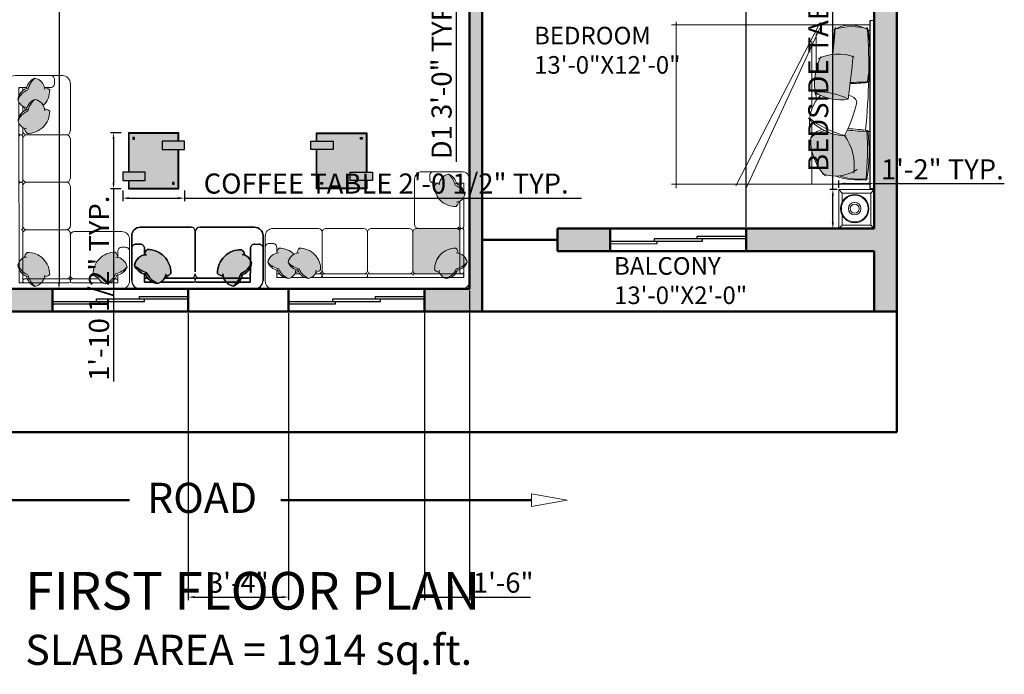
# Model space of a CAD drawing. Units: inches. Extents: x 1913 to 5309, y 1003 to 1733.
# Tile 10 of 23: x 2850 to 3242, y 1003 to 1263. Entities that reach past the tile are written whole.
import ezdxf

# ---------------------------------------------------------------- set-up
doc = ezdxf.new("R2010")
doc.units = ezdxf.units.IN
for name, color, linetype, lineweight in [('0.10', 252, 'Continuous', 9), ('0.15', 34, 'Continuous', 15), ('A-ANNO-DIMS', 2, 'Continuous', 18), ('A-ANNO-SYMB', 1, 'Continuous', 18), ('A-ANNO-TEXT', 7, 'Continuous', 18), ('A-AREA-IDEN', 3, 'Continuous', 18), ('A-DOOR', 4, 'Continuous', 25), ('A-FLOR-PATT', 252, 'Continuous', 13), ('A-FURN', 8, 'Continuous', 18), ('A-FURN-PATT', 8, 'Continuous', 13), ('A-GLAZ', 5, 'Continuous', 25), ('A-WALL', 7, 'Continuous', 50)]:
    doc.layers.add(name, color=color, linetype=linetype, lineweight=lineweight)
doc.layers.add('MOBIL', color=7, linetype='Continuous')
doc.styles.get("Standard").update_dxf_attribs({"font": 'arial.ttf'})
doc.dimstyles.new('ISO-25', dxfattribs={"dimtxt": 8, "dimasz": 2.5, "dimexe": 1.25, "dimexo": 0.625, "dimtad": 1, "dimdec": 1, "dimlunit": 3, "dimtxsty": 'Standard', "dimcen": 2.5, "dimclrd": 256, "dimclrt": 1, "dimadec": 0, "dimazin": 0, "dimtfac": 1, "dimtdec": 1, "dimtmove": 0, "dimatfit": 3, "dimfxl": 1, "dimarcsym": 0})

# ---------------------------------------------------------------- blocks, each defined once
blk = doc.blocks.new('Mesa de centro Cantria feeling')
at = {"layer": 'MOBIL', "ltscale": 0.2}
h = blk.add_hatch(color=256, dxfattribs=at)
h.set_gradient(color1=(74, 55, 38), color2=(104, 77, 54), one_color=1, tint=0.31, name='CYLINDER')
h.paths.add_polyline_path([(-0.85, -0.3), (-0.7, -0.3), (-0.7, 0.1), (-0.85, 0.1)])
h = blk.add_hatch(color=256, dxfattribs=at)
h.set_gradient(color1=(221, 221, 223), one_color=1, tint=1)
h.paths.add_polyline_path([(-0.15, -0.6), (-0.15, -0.89), (-0.01, -0.89), (-0.01, -0.01), (-0.7, -0.01), (-0.7, -0.3), (-0.85, -0.3), (-0.85, -0.01), (-0.99, -0.01), (-0.99, -0.89), (-0.3, -0.89), (-0.3, -0.6)])
h.paths.add_polyline_path([(-0.112, -0.112), (-0.112, -0.082), (-0.082, -0.082), (-0.082, -0.112)], flags=16)
h.paths.add_polyline_path([(-0.888, -0.788), (-0.888, -0.818), (-0.918, -0.818), (-0.918, -0.788)], flags=16)
h = blk.add_hatch(color=256, dxfattribs=at)
h.set_gradient(color1=(74, 55, 38), color2=(104, 77, 54), one_color=1, tint=0.31, name='CYLINDER')
h.paths.add_polyline_path([(-0.15, -0.6), (-0.3, -0.6), (-0.3, -1), (-0.15, -1)])
for points in [[(-0.85, 0), (-1, 0), (-1, -0.9), (-0.3, -0.9)], [(-0.15, -0.9), (0, -0.9), (0, 0), (-0.7, 0)], [(-0.85, -0.01), (-0.99, -0.01), (-0.99, -0.89), (-0.3, -0.89)], [(-0.15, -0.89), (-0.01, -0.89), (-0.01, -0.01), (-0.7, -0.01)]]:
    blk.add_lwpolyline(points, dxfattribs=at)
for points in [[(-0.85, -0.3), (-0.7, -0.3), (-0.7, 0.1), (-0.85, 0.1)], [(-0.082, -0.082), (-0.112, -0.082), (-0.112, -0.112), (-0.082, -0.112)], [(-0.15, -0.6), (-0.3, -0.6), (-0.3, -1), (-0.15, -1)], [(-0.918, -0.818), (-0.888, -0.818), (-0.888, -0.788), (-0.918, -0.788)]]:
    blk.add_lwpolyline(points, close=True, dxfattribs=at)
blk = doc.blocks.new('camita')
at = {"layer": '0.10'}
for p, q in [((-0.85, -0.045), (0.85, -0.045)), ((-0.805, -0.045), (-0.805, -2.0485)), ((0.805, -0.045), (0.805, -2.0485)), ((-0.8271, -0.521), (0.8464, -1.2932)), ((-0.8271, -0.5476), (0.8236, -1.3992)), ((-0.7161, -0.585), (-0.3554, -0.585)), ((-0.1136, -0.585), (-0.0485, -0.585)), ((-0.638, -0.63), (0.0434, -0.63)), ((0.1749, -0.63), (0.3179, -0.63)), ((0.4739, -0.63), (0.805, -0.63)), ((-0.8354, -2), (0.8464, -2))]:
    blk.add_line(p, q, dxfattribs=at)
blk.add_lwpolyline([(-0.85, -0.0405), (0.85, -0.0405), (0.85, 0), (-0.85, 0)], close=True, dxfattribs=at)
for centre, radius, start, end in [((-0.4574, -0.2364), 0.3443, 147.50996, 213.83359), ((-0.1997, -0.2266), 0.5864, 163.92635, 197.14087), ((-0.3639, -5.8457), 5.7909, 83.80731, 94.12107), ((-0.5104, -1.7232), 1.6781, 80.12554, 98.66187), ((2.3534, -0.0532), 2.5803, 180.10628, 184.38541), ((-1.5443, -0.2452), 1.3333, 359.93941, 7.55329), ((1.5815, -0.2893), 1.3353, 170.38021, 178.99138), ((-1.4396, -0.0609), 1.7117, 352.92911, 0.39592), ((0.4524, -3.0675), 2.9996, 83.90257, 93.67595), ((0.4863, -1.6286), 1.5781, 80.16015, 98.05996), ((0.0294, -0.1377), 0.7262, 342.58415, 6.00484), ((0.1326, -0.1696), 0.6307, 339.92303, 8.74334), ((-0.007, -0.258), 0.0828, 100.01798, 179.73597), ((-0.2931, -1.4378), 1.2903, 61.97485, 77.84351), ((0.3203, -0.3944), 0.4043, 341.45245, 33.45121), ((-0.0543, -0.3633), 0.4542, 159.30257, 206.50263), ((-1.3301, -9.6748), 9.4985, 82.27078, 84.93989), ((0.4585, -0.5454), 0.5842, 151.04555, 184.14969), ((-0.5341, -0.3393), 0.4875, 327.26442, 9.0473), ((-0.1986, -0.2742), 0.5159, 310.73945, 359.05759), ((0.6265, -0.7518), 0.5508, 82.96906, 124.67388), ((-1.8672, -14.986), 14.6323, 84.65974, 85.75157), ((-0.5673, -0.0868), 0.9057, 321.69527, 346.46261), ((-0.4598, 1.4861), 1.9092, 260.95299, 268.65169), ((0.3612, -0.133), 0.5096, 267.25889, 315.29965), ((-0.2002, 0.064), 0.6673, 244.78094, 279.06058), ((0.179, -0.272), 0.3828, 224.52836, 275.22287), ((0.4384, -0.4834), 0.1898, 193.68485, 236.70352), ((0.5707, -0.4317), 0.3145, 192.93877, 221.96363)]:
    blk.add_arc(centre, radius, start, end, dxfattribs=at)
blk = doc.blocks.new('VELADOR')
at = {"layer": '0.15'}
for p, q in [((-0.248, 0), (-0.203, -0.045)), ((0.248, 0), (0.202, -0.045)), ((-0.203, -0.405), (-0.248, -0.45)), ((0.248, -0.45), (0.202, -0.405))]:
    blk.add_line(p, q, dxfattribs=at)
blk.add_lwpolyline([(-0.248, 0), (-0.248, -0.45), (0.248, -0.45), (0.248, 0)], close=True, dxfattribs=at)
blk.add_lwpolyline([(0.092, -0.405), (0.202, -0.405), (0.202, -0.045), (-0.203, -0.045), (-0.203, -0.405), (-0.082, -0.405)], dxfattribs=at)
for radius in [0.18, 0.169, 0.0788, 0.0563]:
    blk.add_circle((0.005, -0.247), radius, dxfattribs=at)
blk = doc.blocks.new('d2 s')
at = {"transparency": 33554687}
h = blk.add_hatch(color=256, dxfattribs=at)
h.dxf.hatch_style = 1
h.paths.add_polyline_path([(3953.01, 1202.6, 0.213835), (3948.73, 1198.21, 0.233217), (3951.28, 1195.23, 0.122039), (3952.62, 1192.95, 0.425972), (3962.37, 1202.51, 0.156703), (3960.25, 1203.55), (3960.12, 1203.55, 0.310469), (3955.94, 1207.57, 0.147724)])
h = blk.add_hatch(color=256, dxfattribs=at)
h.dxf.hatch_style = 1
h.paths.add_polyline_path([(3953.9, 1162.75, -0.084911), (3952.59, 1164.92, -0.046133), (3950.85, 1165.51), (3950.85, 1171.8, -0.039409), (3951.63, 1172.02, -0.165523), (3952.68, 1174.28, -0.42585), (3962.24, 1164.53, -0.121928), (3959.96, 1163.19, -0.027403), (3959.75, 1162.75)])
h.paths.add_polyline_path([(3949.17, 1166.48), (3949.17, 1170.75, -0.097704), (3950.85, 1171.8), (3950.85, 1165.51, -0.04873)])
h.paths.add_polyline_path([(3947.62, 1167.84, -0.16488), (3949.17, 1170.75), (3949.17, 1166.48, -0.051917)])
h.paths.add_polyline_path([(3956, 1161.07, -0.090388), (3953.9, 1162.75), (3959.75, 1162.75, -0.136035), (3958.07, 1161.07)])
blk.add_line((3946.53, 1205.25), (3946.53, 1159.36), dxfattribs=at)
for p, q in [((3949.84, 1161.07), (3950.18, 1161.07)), ((3964.47, 1159.37), (3964.46, 1157.65))]:
    blk.add_line(p, q)
for points in [[(3955.94, 1207.57, 0.147724), (3953.01, 1202.6, 0.213355), (3948.73, 1198.22, -0.213355), (3953.01, 1202.6, -0.147724), (3955.94, 1207.57, 0.249545), (3952.4, 1203.17, -0.249545), (3955.93, 1207.59, -0.356779), (3960.22, 1202.7, 0.356779), (3955.94, 1207.57)], [(3948.72, 1198.23, 0.306333), (3952.42, 1194.91, -0.306333), (3948.72, 1198.23, -0.306674), (3952.79, 1203.29, 0.306674), (3948.72, 1198.23)], [(3952.62, 1192.95, 0.425972), (3962.37, 1202.51, 0.165552), (3960.12, 1203.57, -0.165552), (3962.37, 1202.51, -0.425972), (3952.63, 1192.95, -0.121514), (3951.29, 1195.22, 0.121514), (3952.62, 1192.95)], [(3962.24, 1164.53, 0.425972), (3952.68, 1174.28, 0.165552), (3951.63, 1172.02, -0.165552), (3952.68, 1174.28, -0.425972), (3962.24, 1164.53, -0.121514), (3959.97, 1163.19, 0.121514), (3962.24, 1164.53)], [(3947.62, 1167.84, 0.147724), (3952.59, 1164.92, 0.213355), (3956.97, 1160.64, -0.213355), (3952.59, 1164.92, -0.147724), (3947.62, 1167.84, 0.249545), (3952.02, 1164.3, -0.249545), (3947.61, 1167.84, -0.356779), (3952.49, 1172.13, 0.356779), (3947.62, 1167.84)], [(3956.96, 1160.63, 0.306333), (3960.28, 1164.33, -0.306333), (3956.96, 1160.63, -0.306674), (3951.9, 1164.7, 0.306674), (3956.96, 1160.63)]]:
    blk.add_lwpolyline(points, format="xyb", dxfattribs=at)
for points in [[(3949.93, 1208.66), (3967.86, 1208.66)], [(3964.46, 1205.25), (3964.46, 1206.96)], [(3971.27, 1205.25), (3971.27, 1184.84)], [(3949.17, 1203.55), (3952.49, 1203.55), (3949.17, 1203.55), (3949.17, 1199.96)], [(3950.85, 1202.87), (3950.85, 1202.25)], [(3960.13, 1203.55), (3962.77, 1203.55)], [(3949.17, 1197.14), (3949.17, 1183.83)], [(3950.85, 1195.43), (3950.85, 1183.83)], [(3949.17, 1164.09), (3949.17, 1182.51)], [(3950.99, 1183.17), (3950.65, 1183.17)], [(3950.85, 1161.74), (3950.85, 1182.51)], [(3969.63, 1183.17), (3953.36, 1183.17)], [(3971.25, 1181.39), (3971.25, 1159.35)], [(3949.17, 1161.07), (3949.17, 1164.4), (3949.17, 1161.07), (3952.75, 1161.07)], [(3952.75, 1161.06), (3962.77, 1161.06)], [(3949.93, 1155.95), (3967.86, 1155.95)]]:
    blk.add_lwpolyline(points, close=True, dxfattribs=at)
for points in [[(3962.76, 1208.66, -0.414214), (3964.46, 1206.97, 0.414214)], [(3964.46, 1205.26, -0.414214), (3962.76, 1203.57, 0.414214)], [(3967.85, 1208.66, -0.414212), (3971.25, 1205.26, 0.414212)], [(3950.18, 1203.55, -0.414214), (3950.85, 1202.88, 0.414214)], [(3964.47, 1159.37, 0.414214), (3962.77, 1161.06, -0.414214)], [(3967.85, 1155.95, 0.414212), (3971.25, 1159.35, -0.414212)], [(3962.76, 1155.95, 0.414214), (3964.46, 1157.65, -0.414214)]]:
    blk.add_lwpolyline(points, format="xyb", close=True, dxfattribs=at)
for centre, radius, start, end in [((3949.93, 1205.26), 3.4, 90.0002, 179.9998), ((3949.93, 1205.26), 3.4, 90.0846, 180.0842), ((3949.85, 1183.85), 0.681, 179.1575, 269.1575), ((3949.85, 1182.49), 0.681, 90.8425, 180.8425), ((3950.18, 1183.84), 0.671, 270, 0), ((3950.18, 1183.84), 0.671, 270, 0), ((3950.18, 1182.5), 0.671, 360, 90), ((3950.18, 1182.5), 0.671, 360, 90), ((3952.51, 1184.83), 1.66, 179.4889, 271.234), ((3952.51, 1181.52), 1.66, 88.766, 180.5111), ((3969.59, 1184.83), 1.66, 268.766, 0.5111), ((3969.39, 1181.32), 1.86, 2.0577, 84.9818), ((3969.39, 1181.32), 1.86, 2.0577, 84.9818), ((3969.59, 1184.83), 1.66, 268.7816, 0.5111), ((3949.84, 1161.74), 0.671, 180, 270), ((3950.18, 1161.74), 0.671, 270, 0), ((3949.93, 1159.36), 3.4, 180.0002, 269.9998), ((3949.93, 1159.37), 3.4, 180.0846, 270.0842)]:
    blk.add_arc(centre, radius, start, end, dxfattribs=at)
blk = doc.blocks.new('SOFA 1')
at = {"transparency": 33554687}
h = blk.add_hatch(color=256, dxfattribs=at)
h.dxf.hatch_style = 1
h.paths.add_polyline_path([(3769.65, 1307.6, 0.084911), (3767.15, 1309.12, 0.046133), (3766.46, 1311.13), (3759.18, 1311.13, 0.039409), (3758.92, 1310.24, 0.165523), (3756.31, 1309.02, 0.42585), (3767.59, 1297.95, 0.121928), (3769.15, 1300.58, 0.027403), (3769.65, 1300.83)])
h.paths.add_polyline_path([(3765.34, 1313.08), (3760.4, 1313.08, 0.097704), (3759.18, 1311.13), (3766.46, 1311.13, 0.04873)])
h.paths.add_polyline_path([(3763.76, 1314.88, 0.16488), (3760.4, 1313.08), (3765.34, 1313.08, 0.051917)])
h.paths.add_polyline_path([(3771.6, 1305.17, 0.090388), (3769.65, 1307.6), (3769.65, 1300.83, 0.136035), (3771.6, 1302.77)])
h = blk.add_hatch(color=256, dxfattribs=at)
h.dxf.hatch_style = 1
h.paths.add_polyline_path([(3723.52, 1308.63, 0.147724), (3717.76, 1305.24, 0.310469), (3722.42, 1300.4), (3722.42, 1300.25, 0.156703), (3723.62, 1297.8, 0.425821), (3734.69, 1309.08, 0.121928), (3732.05, 1310.63, 0.233216), (3728.6, 1313.59, 0.213835)])
h = blk.add_hatch(color=256, dxfattribs=at)
h.dxf.hatch_style = 1
h.paths.add_polyline_path([(3769.16, 1235.96, 0.122267), (3767.6, 1238.61, 0.425972), (3756.32, 1227.54, 0.165563), (3758.93, 1226.32, 0.309481), (3763.76, 1221.69, 0.002677), (3763.83, 1221.72, 0.146094), (3767.16, 1227.43, 0.212433), (3772.1, 1232.48, 0.235342)])
h = blk.add_hatch(color=256, dxfattribs=at)
h.dxf.hatch_style = 1
h.paths.add_polyline_path([(3769.16, 1225.36, 0.122267), (3767.6, 1228.01, 0.425972), (3756.32, 1216.94, 0.165563), (3758.93, 1215.72, 0.309481), (3763.76, 1211.09, 0.002677), (3763.83, 1211.12, 0.146094), (3767.16, 1216.83, 0.212433), (3772.1, 1221.88, 0.235342)])
for p, q in [((3720.45, 1316.13), (3773.58, 1316.13)), ((3777.51, 1312.19), (3777.51, 1213.72))]:
    blk.add_line(p, q, dxfattribs=at)
for points in [[(3763.76, 1314.88, -0.147724), (3767.15, 1309.12, -0.213355), (3772.1, 1304.05, 0.213355), (3767.15, 1309.12, 0.147724), (3763.76, 1314.88, -0.249545), (3767.86, 1309.77, 0.249545), (3763.77, 1314.89, 0.356779), (3758.8, 1309.23, -0.356779), (3763.76, 1314.88)], [(3717.76, 1305.24, -0.147724), (3723.52, 1308.63, -0.213355), (3728.59, 1313.59, 0.213355), (3723.52, 1308.63, 0.147724), (3717.76, 1305.24, -0.249545), (3722.86, 1309.34, 0.249545), (3717.75, 1305.25, 0.356779), (3723.4, 1300.28, -0.356779), (3717.76, 1305.24)], [(3734.69, 1309.08, -0.425972), (3723.62, 1297.8, -0.165552), (3722.4, 1300.4, 0.165552), (3723.62, 1297.79, 0.425972), (3734.69, 1309.07, 0.121514), (3732.07, 1310.63, -0.121514), (3734.69, 1309.08)], [(3728.58, 1313.6, -0.306333), (3732.42, 1309.31, 0.306333), (3728.58, 1313.6, 0.306674), (3722.72, 1308.89, -0.306674), (3728.58, 1313.6)], [(3767.6, 1297.95, -0.425972), (3756.31, 1309.01, -0.165552), (3758.92, 1310.24, 0.165552), (3756.31, 1309.02, 0.425972), (3767.59, 1297.95, 0.121514), (3769.14, 1300.57, -0.121514), (3767.6, 1297.95)], [(3772.11, 1304.06, -0.306333), (3767.83, 1300.22, 0.306333), (3772.11, 1304.06, 0.306674), (3767.4, 1309.91, -0.306674), (3772.11, 1304.06)], [(3770.44, 1286.63, -0.414214), (3769.66, 1287.4, 0.414214), (3770.44, 1286.63, 0.414214), (3769.66, 1285.83, -0.414214), (3770.44, 1286.63)], [(3748.01, 1262.99, -0.414214), (3746.05, 1264.95, 0.414214), (3748.01, 1262.97, 0.414213), (3746.05, 1261.01, -0.414213), (3748.01, 1262.99)], [(3770.44, 1262.99, -0.414214), (3769.66, 1263.77, 0.414214), (3770.44, 1262.99, 0.414214), (3769.66, 1262.19, -0.414214), (3770.44, 1262.99)], [(3770.83, 1262.97, -0.414214), (3771.61, 1262.19, 0.414214), (3770.83, 1262.99, 0.414214), (3771.61, 1263.77, -0.414214), (3770.83, 1262.97)], [(3748.01, 1239.35, -0.414214), (3746.05, 1241.31, 0.414214), (3748.01, 1239.33, 0.414213), (3746.05, 1237.37, -0.414213), (3748.01, 1239.35)], [(3767.7, 1239.33, -0.414214), (3769.66, 1237.37, 0.414214), (3767.7, 1239.35, 0.414214), (3769.66, 1241.31, -0.414214), (3767.7, 1239.33)], [(3756.32, 1227.54, -0.425972), (3767.6, 1238.61, -0.121514), (3769.16, 1235.98, 0.121514), (3767.6, 1238.61, 0.425972), (3756.32, 1227.54, 0.165552), (3758.93, 1226.32, -0.165552), (3756.32, 1227.54)], [(3772.1, 1232.5, -0.306674), (3767.41, 1226.64, 0.306674), (3772.1, 1232.5, 0.306333), (3767.84, 1236.34, -0.306333), (3772.1, 1232.5)], [(3770.44, 1239.35, -0.414214), (3769.66, 1240.13, 0.414214), (3770.44, 1239.33, 0.414214), (3769.66, 1238.55, -0.414214), (3770.44, 1239.35)], [(3770.83, 1239.33, -0.414214), (3771.61, 1238.55, 0.414214), (3770.83, 1239.35, 0.414214), (3771.61, 1240.13, -0.414214), (3770.83, 1239.33)], [(3763.78, 1221.67, 0.249545), (3767.87, 1226.78, -0.249545), (3763.76, 1221.69, -0.356779), (3758.81, 1227.32, 0.356779), (3763.77, 1221.68, 0.147724), (3767.16, 1227.43, 0.213355), (3772.11, 1232.51, -0.213355), (3767.16, 1227.43, -0.147724), (3763.78, 1221.67)], [(3756.32, 1216.94, -0.200233), (3759.49, 1224.76, 0.200233), (3756.32, 1216.94, 0.165552), (3758.93, 1215.72, -0.165552), (3756.32, 1216.94)], [(3772.1, 1221.9, -0.306674), (3767.41, 1216.04, 0.306674), (3772.1, 1221.9, -0.213355), (3767.16, 1216.83, -0.147724), (3763.77, 1211.08, 0.147724), (3767.15, 1216.83, 0.213355), (3772.1, 1221.9)], [(3763.76, 1211.09, -0.356779), (3758.81, 1216.72, 0.356779), (3763.76, 1211.09, 0.249545), (3767.87, 1216.18, -0.249545), (3763.76, 1211.09)]]:
    blk.add_lwpolyline(points, format="xyb", dxfattribs=at)
for points in [[(3716.51, 1312.2), (3716.51, 1291.44)], [(3722.42, 1313.08), (3722.42, 1309.23), (3722.42, 1313.08), (3726.57, 1313.08)], [(3723.21, 1311.13), (3723.93, 1311.13)], [(3729.85, 1313.08), (3745.25, 1313.08)], [(3731.82, 1311.13), (3745.25, 1311.13)], [(3746.01, 1312.3), (3746.01, 1288.55)], [(3746.01, 1310.97), (3746.01, 1311.36)], [(3768.11, 1313.08), (3746.78, 1313.08)], [(3768.87, 1311.13), (3746.78, 1311.13)], [(3771.6, 1313.08), (3767.75, 1313.08), (3771.6, 1313.08), (3771.6, 1308.93)], [(3769.66, 1287.39), (3769.65, 1312.3)], [(3771.6, 1313.08), (3771.61, 1233.74)], [(3746.01, 1288.54), (3746.01, 1308.23)], [(3769.65, 1309.43), (3769.65, 1308.71)], [(3722.42, 1300.39), (3722.42, 1297.33)], [(3720.45, 1295.38), (3718.48, 1295.38)], [(3720.45, 1287.5), (3744.09, 1287.5)], [(3747.99, 1286.6), (3767.69, 1286.6)], [(3769.66, 1263.75), (3769.66, 1285.81)], [(3746.02, 1284.63), (3746.02, 1264.94)], [(3769.66, 1277.18), (3769.66, 1263.75)], [(3746.02, 1260.99), (3746.02, 1241.3)], [(3747.99, 1262.97), (3767.69, 1262.97)], [(3769.66, 1240.12), (3769.66, 1262.18)], [(3770.43, 1262.97), (3770.82, 1262.97)], [(3746.02, 1237.36), (3746.02, 1213.74)], [(3747.99, 1239.33), (3767.69, 1239.33)], [(3769.66, 1235.71), (3769.66, 1238.54)], [(3770.43, 1239.33), (3770.82, 1239.33)], [(3769.66, 1225.11), (3769.66, 1227.82)], [(3771.61, 1223.14), (3771.61, 1230.47)], [(3767.76, 1215.72), (3771.61, 1215.72), (3771.61, 1219.84), (3771.61, 1215.72)], [(3769.66, 1216.5), (3769.66, 1217.22)], [(3753.91, 1211.77), (3753.91, 1213.74)], [(3755.86, 1215.72), (3758.92, 1215.72)], [(3749.97, 1209.8), (3773.58, 1209.8)]]:
    blk.add_lwpolyline(points, close=True, dxfattribs=at)
for points in [[(3722.42, 1311.91, 0.414214), (3723.2, 1311.13, -0.414214)], [(3770.43, 1313.08, 0.414214), (3769.65, 1312.3, -0.414214)], [(3771.6, 1312.3, 0.414214), (3770.82, 1313.08, -0.414214)], [(3716.51, 1297.34, 0.414214), (3718.47, 1295.38, -0.414214)], [(3720.44, 1295.38, 0.414214), (3722.4, 1297.34, -0.414214)], [(3716.51, 1291.45, 0.414212), (3720.44, 1287.52, -0.414212)], [(3746.03, 1288.56, 0.414214), (3747.99, 1286.6, 0.414213), (3746.03, 1284.64, -0.414213), (3747.99, 1286.6, -0.414214)], [(3769.66, 1284.64, 0.414214), (3767.7, 1286.6, 0.414214), (3769.66, 1288.56, -0.414214), (3767.7, 1286.6, -0.414214)], [(3769.66, 1261.01, 0.414214), (3767.7, 1262.97, 0.414214), (3769.66, 1264.93, -0.414214), (3767.7, 1262.97, -0.414214)], [(3769.16, 1225.36, 0.071861), (3768.39, 1227.01, -0.071861)], [(3772.13, 1221.9, 0.306333), (3767.84, 1225.74, -0.306333)], [(3746.05, 1213.76, 0.414212), (3749.98, 1209.82, -0.414212)], [(3755.87, 1215.72, 0.414214), (3753.91, 1213.76, -0.414214)], [(3769.66, 1216.52, 0.414214), (3770.44, 1215.74, -0.414214)], [(3770.83, 1215.74, 0.414214), (3771.61, 1216.52, -0.414214)], [(3755.87, 1209.8, -0.414214), (3753.91, 1211.76, 0.414214)]]:
    blk.add_lwpolyline(points, format="xyb", close=True, dxfattribs=at)
for centre, radius, start, end in [((3720.44, 1312.2), 3.93, 90.0002, 179.9998), ((3720.44, 1312.19), 3.94, 89.9158, 179.9154), ((3773.58, 1312.2), 3.93, 0.0002, 89.9998), ((3773.57, 1312.19), 3.94, 359.9158, 89.9154), ((3744.09, 1309.21), 1.92, 358.766, 90.5111), ((3745.22, 1312.29), 0.789, 0.8425, 90.8425), ((3745.24, 1311.91), 0.777, 270, 0), ((3745.24, 1311.91), 0.777, 270, 0), ((3746.8, 1312.29), 0.789, 89.1575, 179.1575), ((3746.79, 1311.91), 0.777, 180, 270), ((3746.79, 1311.91), 0.777, 180, 270), ((3747.93, 1309.21), 1.92, 89.4889, 181.234), ((3768.87, 1312.3), 0.777, 360, 90), ((3768.87, 1311.91), 0.777, 270, 0), ((3744.08, 1289.48), 1.96, 270, 360), ((3744.08, 1289.48), 1.96, 270, 360), ((3773.58, 1213.73), 3.93, 270.0002, 359.9998), ((3773.59, 1213.73), 3.93, 269.9156, 359.9152)]:
    blk.add_arc(centre, radius, start, end, dxfattribs=at)
blk = doc.blocks.new('*D48')
at = {"layer": 'A-ANNO-DIMS', "color": 0, "lineweight": -2, "transparency": 16777216}
for p, q in [((2859.93, 1599.96), (2867.23, 1599.96)), ((2865.98, 1597.46), (2865.98, 1158.43)), ((2859.93, 1155.93), (2867.23, 1155.93))]:
    blk.add_line(p, q, dxfattribs=at)
at = {"layer": 'A-ANNO-DIMS', "color": 0, "transparency": 16777216}
for points in [[(2865.56, 1597.46), (2866.39, 1597.46), (2865.98, 1599.96)], [(2865.56, 1158.43), (2866.39, 1158.43), (2865.98, 1155.93)]]:
    blk.add_solid(points, dxfattribs=at)
at = {"layer": 'Defpoints', "color": 0, "transparency": 16777216}
for p in [(2859.31, 1599.96), (2859.31, 1155.93), (2865.98, 1155.93)]:
    blk.add_point(p, dxfattribs=at)
at = {"layer": 'A-ANNO-DIMS', "color": 0, "transparency": 16777216, "insert": (2861.26, 1377.95), "char_height": 8, "attachment_point": 5, "rotation": 90}
blk.add_mtext("37'", dxfattribs=at)
blk = doc.blocks.new('WIN-54')
for p, q in [((0, 54), (0, 35)), ((1, 54), (1, 17)), ((1, 36), (2, 36)), ((2, 36), (2, 0)), ((0, 35), (1, 35)), ((1, 17), (2, 17)), ((2, 19), (3, 19)), ((3, 19), (3, 0))]:
    blk.add_line(p, q)
blk = doc.blocks.new('*D55')
at = {"layer": 'A-ANNO-DIMS', "lineweight": -2, "transparency": 16777216}
for p, q in [((3173.87, 1195.51), (3173.87, 1356.99)), ((3173.87, 1182.46), (3173.87, 1193.01))]:
    blk.add_line(p, q, dxfattribs=at)
at = {"layer": 'A-ANNO-DIMS', "color": 0, "lineweight": -2, "transparency": 16777216}
for p, q in [((3175.58, 1195.51), (3172.62, 1195.51)), ((3175.58, 1179.96), (3172.62, 1179.96))]:
    blk.add_line(p, q, dxfattribs=at)
at = {"layer": 'A-ANNO-DIMS', "transparency": 16777216}
for points in [[(3173.45, 1193.01), (3174.29, 1193.01), (3173.87, 1195.51)], [(3173.45, 1182.46), (3174.29, 1182.46), (3173.87, 1179.96)]]:
    blk.add_solid(points, dxfattribs=at)
at = {"layer": 'Defpoints', "color": 0, "transparency": 16777216}
for p in [(3173.87, 1195.51), (3176.2, 1195.51), (3176.2, 1179.96)]:
    blk.add_point(p, dxfattribs=at)
at = {"layer": 'A-ANNO-DIMS', "color": 1, "transparency": 16777216, "insert": (3169.1, 1277.5), "char_height": 8, "attachment_point": 5, "rotation": 90}
blk.add_mtext('BEDSIDE TABLE 1\'-3 1/2" TYP.', dxfattribs=at)
blk = doc.blocks.new('*D56')
at = {"layer": 'A-ANNO-DIMS', "color": 0, "lineweight": -2, "transparency": 16777216}
for p, q in [((3176.2, 1196.14), (3176.2, 1199.1)), ((3190.34, 1196.14), (3190.34, 1199.1))]:
    blk.add_line(p, q, dxfattribs=at)
at = {"layer": 'A-ANNO-DIMS', "lineweight": -2, "transparency": 16777216}
for p, q in [((3178.7, 1197.85), (3187.84, 1197.85)), ((3190.34, 1197.85), (3242.1, 1197.85))]:
    blk.add_line(p, q, dxfattribs=at)
at = {"layer": 'A-ANNO-DIMS', "transparency": 16777216}
for points in [[(3178.7, 1198.26), (3178.7, 1197.43), (3176.2, 1197.85)], [(3187.84, 1198.26), (3187.84, 1197.43), (3190.34, 1197.85)]]:
    blk.add_solid(points, dxfattribs=at)
at = {"layer": 'Defpoints', "color": 0, "transparency": 16777216}
for p in [(3176.2, 1195.51), (3190.34, 1197.85), (3190.34, 1195.51)]:
    blk.add_point(p, dxfattribs=at)
at = {"layer": 'A-ANNO-DIMS', "color": 1, "transparency": 16777216, "insert": (3217.47, 1202.49), "char_height": 8, "attachment_point": 5}
blk.add_mtext('1\'-2" TYP.', dxfattribs=at)
blk = doc.blocks.new('*D63')
at = {"layer": 'A-ANNO-DIMS', "color": 0, "lineweight": -2, "transparency": 16777216}
for p, q in [((2891.35, 1195.13), (2891.35, 1190.82)), ((2915.89, 1195.13), (2915.89, 1190.82))]:
    blk.add_line(p, q, dxfattribs=at)
at = {"layer": 'A-ANNO-DIMS', "lineweight": -2, "transparency": 16777216}
for p, q in [((2893.85, 1192.07), (2913.39, 1192.07)), ((2915.89, 1192.07), (3073.9, 1192.07))]:
    blk.add_line(p, q, dxfattribs=at)
at = {"layer": 'A-ANNO-DIMS', "transparency": 16777216}
for points in [[(2893.85, 1192.48), (2893.85, 1191.65), (2891.35, 1192.07)], [(2913.39, 1192.48), (2913.39, 1191.65), (2915.89, 1192.07)]]:
    blk.add_solid(points, dxfattribs=at)
at = {"layer": 'Defpoints', "color": 0, "transparency": 16777216}
for p in [(2891.35, 1195.75), (2915.89, 1195.75), (2915.89, 1192.07)]:
    blk.add_point(p, dxfattribs=at)
at = {"layer": 'A-ANNO-DIMS', "color": 1, "transparency": 16777216, "insert": (2996.15, 1196.83), "char_height": 8, "attachment_point": 5}
blk.add_mtext('COFFEE TABLE 2\'-0 1/2" TYP.', dxfattribs=at)
blk = doc.blocks.new('*D64')
at = {"layer": 'A-ANNO-DIMS', "color": 0, "lineweight": -2, "transparency": 16777216}
for p, q in [((2890.72, 1218.06), (2886.42, 1218.06)), ((2890.72, 1195.75), (2886.42, 1195.75))]:
    blk.add_line(p, q, dxfattribs=at)
at = {"layer": 'A-ANNO-DIMS', "lineweight": -2, "transparency": 16777216}
for p, q in [((2887.67, 1215.56), (2887.67, 1198.25)), ((2887.67, 1195.75), (2887.67, 1119.13))]:
    blk.add_line(p, q, dxfattribs=at)
at = {"layer": 'A-ANNO-DIMS', "transparency": 16777216}
for points in [[(2887.25, 1215.56), (2888.08, 1215.56), (2887.67, 1218.06)], [(2887.25, 1198.25), (2888.08, 1198.25), (2887.67, 1195.75)]]:
    blk.add_solid(points, dxfattribs=at)
at = {"layer": 'Defpoints', "color": 0, "transparency": 16777216}
for p in [(2891.35, 1218.06), (2887.67, 1195.75), (2891.35, 1195.75)]:
    blk.add_point(p, dxfattribs=at)
at = {"layer": 'A-ANNO-DIMS', "color": 1, "transparency": 16777216, "insert": (2882.91, 1156.19), "char_height": 8, "attachment_point": 5, "rotation": 90}
blk.add_mtext('1\'-10 1/2" TYP.', dxfattribs=at)
blk = doc.blocks.new('*D71')
at = {"layer": 'A-ANNO-DIMS', "color": 0, "lineweight": -2, "transparency": 16777216}
for p, q in [((3028.71, 1311.96), (3022.69, 1311.96)), ((3028.71, 1275.96), (3022.69, 1275.96))]:
    blk.add_line(p, q, dxfattribs=at)
at = {"layer": 'A-ANNO-DIMS', "lineweight": -2, "transparency": 16777216}
for p, q in [((3023.94, 1309.46), (3023.94, 1278.46)), ((3023.94, 1275.96), (3023.94, 1206.46))]:
    blk.add_line(p, q, dxfattribs=at)
at = {"layer": 'A-ANNO-DIMS', "transparency": 16777216}
for points in [[(3023.52, 1309.46), (3024.36, 1309.46), (3023.94, 1311.96)], [(3023.52, 1278.46), (3024.36, 1278.46), (3023.94, 1275.96)]]:
    blk.add_solid(points, dxfattribs=at)
at = {"layer": 'Defpoints', "color": 0, "transparency": 16777216}
for p in [(3029.34, 1311.96), (3023.94, 1275.96), (3029.34, 1275.96)]:
    blk.add_point(p, dxfattribs=at)
at = {"layer": 'A-ANNO-DIMS', "color": 1, "transparency": 16777216, "insert": (3019.23, 1239.96), "char_height": 8, "attachment_point": 5, "rotation": 90}
blk.add_mtext('D1 3\'-0" TYP.', dxfattribs=at)
blk = doc.blocks.new('*D123')
at = {"layer": 'A-ANNO-DIMS', "color": 0, "lineweight": -2, "transparency": 16777216}
for p, q in [((3011.34, 1155.34), (3011.34, 1032.04)), ((3029.34, 1155.34), (3029.34, 1032.04))]:
    blk.add_line(p, q, dxfattribs=at)
at = {"layer": 'A-ANNO-DIMS', "lineweight": -2, "transparency": 16777216}
for p, q in [((3013.84, 1033.29), (3026.84, 1033.29)), ((3029.34, 1033.29), (3053.6, 1033.29))]:
    blk.add_line(p, q, dxfattribs=at)
at = {"layer": 'A-ANNO-DIMS', "transparency": 16777216}
for points in [[(3013.84, 1033.7), (3013.84, 1032.87), (3011.34, 1033.29)], [(3026.84, 1033.7), (3026.84, 1032.87), (3029.34, 1033.29)]]:
    blk.add_solid(points, dxfattribs=at)
at = {"layer": 'Defpoints', "color": 0, "transparency": 16777216}
for p in [(3011.34, 1155.96), (3029.34, 1155.96), (3029.34, 1033.29)]:
    blk.add_point(p, dxfattribs=at)
at = {"layer": 'A-ANNO-DIMS', "color": 1, "transparency": 16777216, "insert": (3042.72, 1038), "char_height": 8, "attachment_point": 5}
blk.add_mtext('1\'-6"', dxfattribs=at)
blk = doc.blocks.new('*D124')
at = {"layer": 'A-ANNO-DIMS', "color": 0, "lineweight": -2, "transparency": 16777216}
for p, q in [((2917.34, 1146.34), (2917.34, 1032.04)), ((2957.34, 1146.34), (2957.34, 1032.04))]:
    blk.add_line(p, q, dxfattribs=at)
at = {"layer": 'A-ANNO-DIMS', "lineweight": -2, "transparency": 16777216}
blk.add_line((2919.84, 1033.29), (2954.84, 1033.29), dxfattribs=at)
at = {"layer": 'A-ANNO-DIMS', "transparency": 16777216}
for points in [[(2919.84, 1033.7), (2919.84, 1032.87), (2917.34, 1033.29)], [(2954.84, 1033.7), (2954.84, 1032.87), (2957.34, 1033.29)]]:
    blk.add_solid(points, dxfattribs=at)
at = {"layer": 'Defpoints', "color": 0, "transparency": 16777216}
for p in [(2917.34, 1146.96), (2957.34, 1146.96), (2957.34, 1033.29)]:
    blk.add_point(p, dxfattribs=at)
at = {"layer": 'A-ANNO-DIMS', "color": 1, "transparency": 16777216, "insert": (2937.34, 1038), "char_height": 8, "attachment_point": 5}
blk.add_mtext('3\'-4"', dxfattribs=at)
blk = doc.blocks.new('*D126')
at = {"layer": 'A-ANNO-DIMS', "color": 0, "lineweight": -2, "transparency": 16777216}
for p, q in [((3139.34, 1180.59), (3139.34, 1724.21)), ((3190.34, 1180.59), (3190.34, 1724.21))]:
    blk.add_line(p, q, dxfattribs=at)
at = {"layer": 'A-ANNO-DIMS', "lineweight": -2, "transparency": 16777216}
blk.add_line((3141.84, 1722.96), (3187.84, 1722.96), dxfattribs=at)
at = {"layer": 'A-ANNO-DIMS', "transparency": 16777216}
for points in [[(3141.84, 1723.38), (3141.84, 1722.55), (3139.34, 1722.96)], [(3187.84, 1723.38), (3187.84, 1722.55), (3190.34, 1722.96)]]:
    blk.add_solid(points, dxfattribs=at)
at = {"layer": 'Defpoints', "color": 0, "transparency": 16777216}
for p in [(3190.34, 1722.96), (3139.34, 1179.96), (3190.34, 1179.96)]:
    blk.add_point(p, dxfattribs=at)
at = {"layer": 'A-ANNO-DIMS', "color": 1, "transparency": 16777216, "insert": (3164.84, 1727.68), "char_height": 8, "attachment_point": 5}
blk.add_mtext('4\'-3"', dxfattribs=at)

msp = doc.modelspace()

# ---------------------------------------------------------------- hatches: boundary and pattern name
at = {"layer": 'A-FLOR-PATT'}
h = msp.add_hatch(color=256, dxfattribs=at)
h.dxf.hatch_style = 1
h.paths.add_polyline_path([(2841.34, 1686.96), (2683.34, 1686.96), (2683.34, 1625.96), (2692.34, 1625.96), (2692.34, 1677.96), (2836.34, 1677.96), (2836.34, 1554.96), (2841.34, 1554.96), (2841.34, 1599.96), (2859.31, 1599.96), (2859.31, 1608.96), (2841.34, 1608.96)])
h.paths.add_polyline_path([(3034.34, 1625.46), (3029.34, 1625.46), (3029.34, 1608.96), (2955.31, 1608.96), (2955.31, 1599.96), (3029.34, 1599.96), (3029.34, 1528.96), (3034.34, 1528.96)])
h.paths.add_polyline_path([(3199.34, 1686.96), (3029.34, 1686.96), (3029.34, 1661.46), (3034.34, 1661.46), (3034.34, 1677.96), (3190.34, 1677.96), (3190.34, 1492.96), (3029.34, 1492.96), (3029.34, 1487.96), (3158.34, 1487.96), (3158.34, 1464.96), (3163.34, 1464.96), (3163.34, 1487.96), (3199.34, 1487.96)])
h.paths.add_polyline_path([(3099.34, 1400.96), (3163.34, 1400.96), (3163.34, 1428.96), (3158.34, 1428.96), (3158.34, 1405.96), (3029.34, 1405.96), (3029.34, 1311.96), (3034.34, 1311.96), (3034.34, 1323.96), (3058.34, 1323.96), (3058.34, 1328.96), (3034.34, 1328.96), (3034.34, 1400.96), (3094.34, 1400.96), (3094.34, 1358.96), (3099.34, 1358.96)])
h.paths.add_polyline_path([(3199.34, 1405.96), (3187.34, 1405.96), (3187.34, 1400.96), (3190.34, 1400.96), (3190.34, 1328.96), (3094.34, 1328.96), (3094.34, 1323.96), (3190.34, 1323.96), (3190.34, 1299.96), (3190.34, 1179.96), (3176.2, 1179.96), (3139.34, 1179.96), (3139.34, 1170.96), (3190.34, 1170.96), (3190.34, 1146.96), (3199.34, 1146.96)])
h.paths.add_polyline_path([(3085.34, 1179.96), (3064.34, 1179.96), (3064.34, 1170.96), (3085.34, 1170.96)])
h.paths.add_polyline_path([(3029.34, 1158.98), (3029.34, 1199.59, 0.414216), (3026.32, 1202.59), (3010.47, 1202.59, 0.414214), (3007.47, 1199.59), (3007.47, 1181.52, 0.46174), (3009.2, 1180.04), (3026.11, 1180.04, 0.414263), (3025.52, 1179.45), (3025.52, 1162.57, 0.41435), (3026.11, 1161.97), (3007.38, 1161.97, 0.41842), (3006.78, 1161.36, 0.785879), (3005.87, 1162.09, 0.298637), (3006.77, 1163.46), (3006.77, 1178.53, 0.414214), (3005.27, 1180.02), (2990.22, 1180.02, 0.416116), (2988.72, 1178.51, 0.414208), (2987.21, 1180.02), (2987.2, 1180.02, -0.413869), (2988.7, 1178.52, -0.412492), (2990.21, 1180.02), (2990.21, 1180.03), (3005.27, 1180.02, -0.414213), (3006.77, 1178.53, -0.414214), (3008.27, 1180.02), (3008.14, 1180.27, -0.252555), (3007.47, 1181.52), (3007.45, 1181.51), (3007.47, 1199.59, -0.414214), (3010.47, 1202.59), (3026.33, 1202.59, -0.414214), (3029.34, 1199.59), (3029.34, 1275.96), (3034.34, 1275.96), (3034.34, 1146.96), (3011.34, 1146.96), (3011.34, 1155.96), (2951.06, 1155.96, -0.414214), (2948.06, 1158.97), (2948.06, 1158.97, 0.421637), (2951.14, 1155.96), (3026.4, 1155.96, 0.407251)])
h.paths.add_polyline_path([(2845.34, 1275.96), (2836.34, 1275.96), (2836.34, 1233.96), (2845.34, 1233.96), (2845.34, 1237.71)])
h.paths.add_polyline_path([(2845.34, 1173.96), (2836.34, 1173.96), (2836.34, 1146.96), (2863.34, 1146.96), (2863.34, 1155.93), (2848.48, 1155.93, -0.414214), (2845.34, 1159.07)])
h.paths.add_polyline_path([(2841.34, 1356.96), (2836.34, 1356.96), (2836.34, 1328.96), (2793.34, 1328.96), (2793.34, 1405.96), (2841.34, 1405.96), (2841.34, 1470.96), (2836.34, 1470.96), (2836.34, 1410.96), (2769.34, 1410.96), (2769.34, 1513.96), (2836.34, 1513.96), (2836.34, 1506.96), (2841.34, 1506.96), (2841.34, 1518.96), (2764.34, 1518.96), (2764.34, 1405.96), (2788.34, 1405.96), (2788.34, 1328.96), (2692.34, 1328.96), (2692.34, 1340.96), (2683.34, 1340.96), (2683.34, 1323.96), (2841.34, 1323.96)])
h.paths.add_polyline_path([(2692.34, 1513.96), (2734.34, 1513.96), (2734.34, 1518.96), (2692.34, 1518.96), (2692.34, 1571.96), (2683.34, 1571.96), (2683.34, 1420.96), (2683.34, 1364.96), (2692.34, 1364.96), (2692.34, 1405.96), (2734.34, 1405.96), (2734.34, 1410.96), (2692.34, 1410.96)])
at = {"layer": 'A-FURN-PATT'}
h = msp.add_hatch(color=256, dxfattribs=at)
h.dxf.hatch_style = 1
h.paths.add_polyline_path([(3173.91, 1249.25, -0.113891), (3181.91, 1248.39, -0.006967), (3180.83, 1238.02, -0.016701), (3187.61, 1238.29, 0.015442), (3188.18, 1242.33, 0.01851), (3187.65, 1259.2, 0.020657), (3186.66, 1259.71, 0.131047), (3174.76, 1259.33, -0.004387)])
h.paths.add_polyline_path([(3179.64, 1219.16, -0.011742), (3178.57, 1217.03, -0.175864), (3182.33, 1202.71, -0.098488), (3176.39, 1200.9, 0.094792), (3187.07, 1199.68, 0.040212), (3187.45, 1218.65, -0.029051)])
h = msp.add_hatch(color=256, dxfattribs=at)
h.dxf.hatch_style = 1
h.paths.add_polyline_path([(3166.77, 1234.13, 0.181694), (3180, 1231.43, 0.011408), (3181.91, 1248.39, 0.189536), (3168.83, 1247.87, 0.134508)])
h.paths.add_polyline_path([(3178.67, 1216.89, -0.104045), (3170.57, 1218.96, 0.127326), (3165.06, 1216.1, 0.202559), (3170.44, 1201.43, 0.194952), (3182.33, 1202.71, 0.173835)])

# ---------------------------------------------------------------- linework, layer by layer
at = {"layer": 'A-ANNO-SYMB'}
msp.add_lwpolyline([(3068.16, 1071.84), (3054, 1074.39), (3054, 1069.29)], close=True, dxfattribs=at)
at = {"layer": 'A-WALL'}
for p, q in [((3199.34, 1405.96), (3199.34, 1098.96)), ((3190.34, 1323.96), (3190.34, 1179.96)), ((3029.34, 1275.96), (3029.34, 1155.96)), ((3034.34, 1275.96), (3034.34, 1146.96)), ((3064.34, 1179.96), (3190.34, 1179.96)), ((3064.34, 1179.96), (3064.34, 1170.96)), ((3085.34, 1179.96), (3085.34, 1170.96)), ((3139.34, 1179.96), (3139.34, 1170.96)), ((3064.34, 1175.46), (3034.34, 1175.46)), ((3064.34, 1170.96), (3190.34, 1170.96)), ((3190.34, 1170.96), (3190.34, 1146.96)), ((2845.34, 1155.96), (3029.34, 1155.96)), ((2863.34, 1155.96), (2863.34, 1146.96)), ((2917.34, 1155.96), (2917.34, 1146.96)), ((2957.34, 1155.96), (2957.34, 1146.96)), ((3011.34, 1155.96), (3011.34, 1146.96)), ((2836.34, 1146.96), (3199.34, 1146.96)), ((3199.34, 1098.96), (2647.34, 1098.96)), ((2794.16, 1071.84), (2893.98, 1071.84)), ((3054, 1071.84), (2954.18, 1071.84))]:
    msp.add_line(p, q, dxfattribs=at)

# ---------------------------------------------------------------- block references
at = {"layer": 'A-DOOR', "xscale": 0.9914887765283156, "yscale": 0.9914887765283156, "zscale": 0.9914887765283156, "rotation": 90}
msp.add_blockref('d2 s', (4093.29, -2756.97), dxfattribs=at)
at = {"layer": 'A-FURN'}
for name, p, xscale, yscale, zscale, rotation in [('camita', (3190.34, 1229.36), 39.375, 39.375, 39.375, 270), ('SOFA 1', (5861.8, 2206.9), 0.7985303345031592, 0.7985303345031592, 0.7985303345031592, 180), ('Mesa de centro Cantria feeling', (2913.66, 1195.75), 22.3138190187957, 22.3138190187957, 22.3138190187957, 270), ('Mesa de centro Cantria feeling', (2968.38, 1195.75), -22.3138190187957, 22.3138190187957, 22.3138190187957, 90), ('SOFA 1', (2023.28, 4043.51), 0.7644053585719659, 0.7644053585719659, 0.7644053585719659, 270), ('VELADOR', (3190.34, 1187.74), -31.41542173157097, 31.41542173157097, 31.41542173157097, 269.9999999999999)]:
    msp.add_blockref(name, p, dxfattribs=dict(at, xscale=xscale, yscale=yscale, zscale=zscale, rotation=rotation))
at = {"layer": 'A-GLAZ'}
for p, rotation in [((3138.96, 1173.98), 90.04407578688497), ((2916.96, 1149.98), 90.04407578688559), ((3010.96, 1149.98), 90.04407578688559)]:
    msp.add_blockref('WIN-54', p, dxfattribs=dict(at, rotation=rotation))

# ---------------------------------------------------------------- texts
at = {"layer": 'A-ANNO-TEXT', "attachment_point": 1}
for s, width, insert, char_height in [('  ROAD', 86.9528, (2893.71, 1078.77), 12), ('FIRST FLOOR PLAN\\P{\\H0.8x;SLAB AREA = 1914 sq.ft.}', 253.2094, (2852.55, 1043.3), 15)]:
    msp.add_mtext_dynamic_manual_height_columns(s, width=width, gutter_width=12.5, heights=[0], dxfattribs=dict(at, insert=insert, char_height=char_height))
at = {"layer": 'A-AREA-IDEN', "char_height": 7, "attachment_point": 1}
for s, insert in [('BEDROOM\\P13\'-0"X12\'-0"', (3055.01, 1260.26)), ('BALCONY\\P13\'-0"X2\'-0"', (3086.83, 1168.58))]:
    msp.add_mtext_dynamic_manual_height_columns(s, width=86.9528, gutter_width=12.5, heights=[0], dxfattribs=dict(at, insert=insert))

# ---------------------------------------------------------------- dimensions: what is measured, and where the dimension line sits
at = {"layer": 'A-ANNO-DIMS'}
for base, p1, p2, picture, middle in [((3190.34, 1722.96), (3139.34, 1179.96), (3190.34, 1179.96), '*D126', (3164.84, 1727.68)), ((3029.34, 1033.29), (3011.34, 1155.96), (3029.34, 1155.96), '*D123', (3042.72, 1038)), ((2957.34, 1033.29), (2917.34, 1146.96), (2957.34, 1146.96), '*D124', (2937.34, 1038))]:
    dim = msp.add_linear_dim(base=base, p1=p1, p2=p2, dimstyle='ISO-25', override={"dimdec": 1, "dimlfac": 1, "dimrnd": 0, "dimzin": 1, "dimdsep": 46, "dimlunit": 4, "dimfrac": 2}, dxfattribs=at)
    dim.commit()
    dim.dimension.update_dxf_attribs({"geometry": picture, "text_midpoint": middle})
dim = msp.add_linear_dim(base=(2865.98, 1155.93), p1=(2859.31, 1599.96), p2=(2859.31, 1155.93), angle=90, dimstyle='ISO-25', override={"dimclrd": 0, "dimclre": 0, "dimclrt": 0}, dxfattribs=at)
dim.commit()
dim.dimension.update_dxf_attribs({"geometry": '*D48', "text_midpoint": (2861.26, 1377.95)})
for base, p1, p2, angle, text, picture, middle in [((3173.869, 1195.5147), (3176.2016, 1179.9641), (3176.2016, 1195.5147), 90, 'BEDSIDE TABLE <> TYP.', '*D55', (3169.1049, 1277.5046)), ((3023.94, 1275.96), (3029.34, 1311.96), (3029.34, 1275.96), 270, 'D1 <> TYP.', '*D71', (3019.23, 1239.96)), ((2887.67, 1195.75), (2891.35, 1218.06), (2891.35, 1195.75), 270, '<> TYP.', '*D64', (2882.91, 1156.19))]:
    dim = msp.add_linear_dim(base=base, p1=p1, p2=p2, angle=angle, text=text, dimstyle='ISO-25', override={"dimdec": 1, "dimrnd": 0, "dimzin": 1, "dimlunit": 4, "dimfrac": 2}, dxfattribs=at)
    dim.commit()
    dim.dimension.update_dxf_attribs({"geometry": picture, "text_midpoint": middle})
for base, p1, p2, text, picture, middle in [((2915.89, 1192.07), (2891.35, 1195.75), (2915.89, 1195.75), 'COFFEE TABLE <> TYP.', '*D63', (2996.15, 1196.83)), ((3190.34, 1197.85), (3176.2, 1195.51), (3190.34, 1195.51), '<> TYP.', '*D56', (3217.47, 1202.49))]:
    dim = msp.add_linear_dim(base=base, p1=p1, p2=p2, text=text, dimstyle='ISO-25', override={"dimdec": 1, "dimrnd": 0, "dimzin": 1, "dimlunit": 4, "dimfrac": 2}, dxfattribs=at)
    dim.commit()
    dim.dimension.update_dxf_attribs({"geometry": picture, "text_midpoint": middle})

doc.saveas('drawing.dxf')
